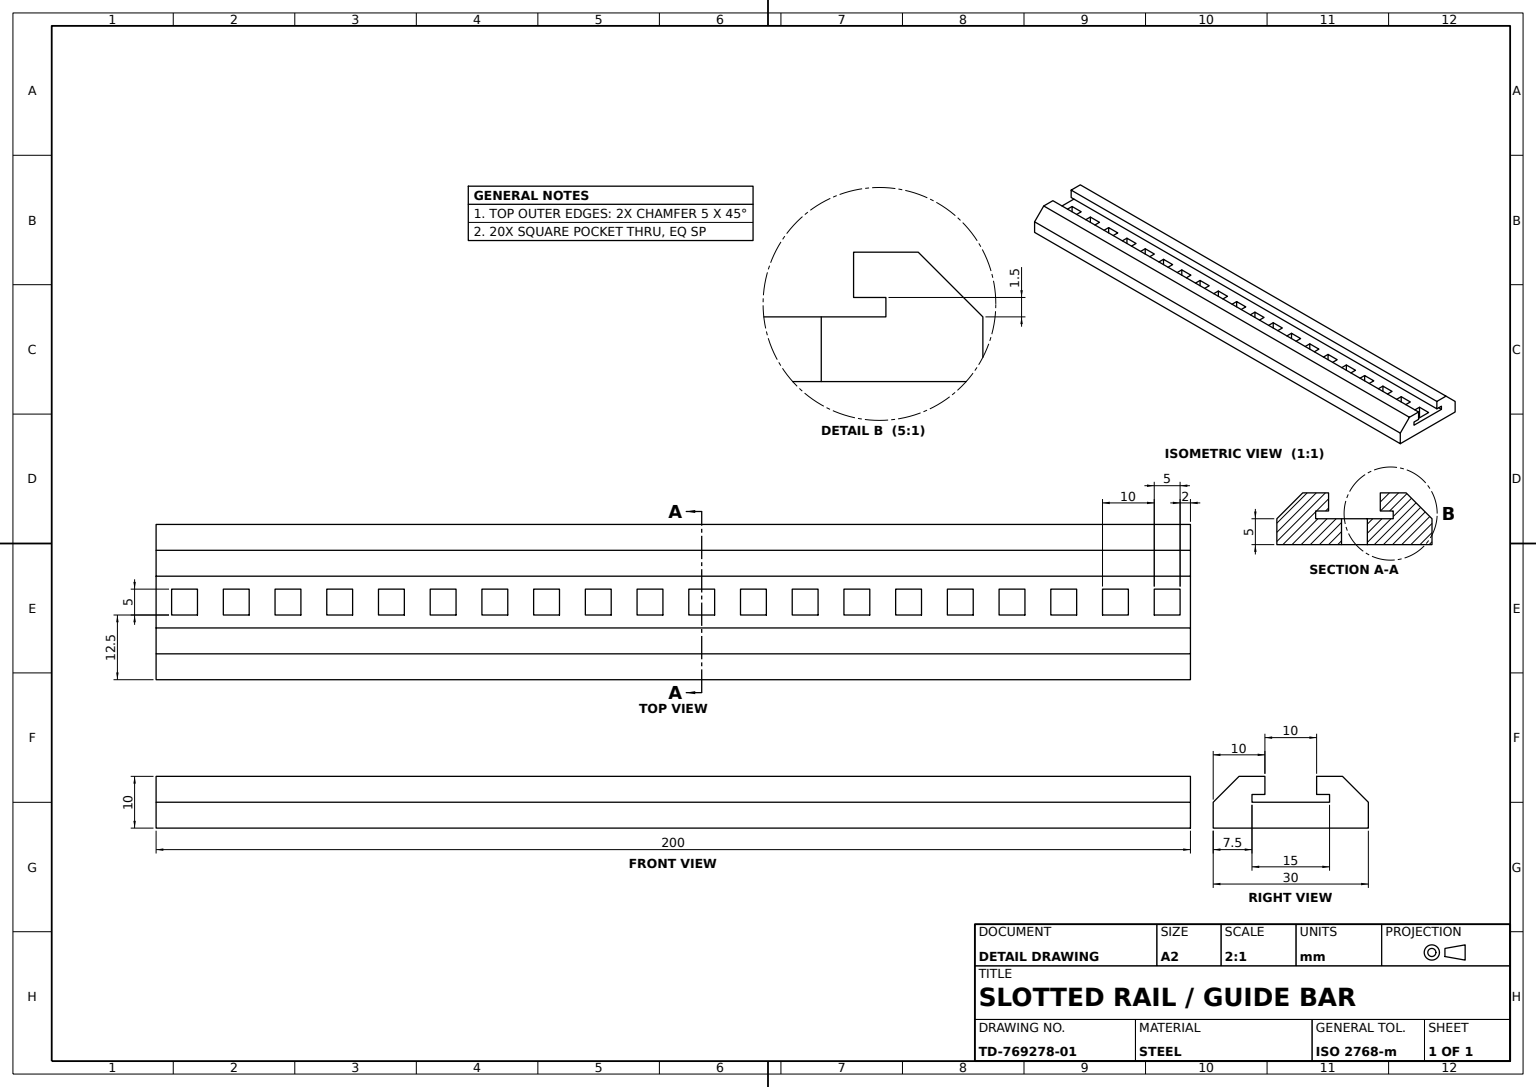
from build123d import *

# Parameters (mm, degrees)
TRACK_PROFILE_SKETCH_W            = 30
TRACK_PROFILE_SKETCH_H            = 10
TRACK_BODY_200MM_DEPTH            = 100
EDGE_CHAMFER_5MM_SIZE             = 5
GUIDE_GROOVE_SKETCH_W             = 10
GUIDE_GROOVE_SKETCH_H             = 200
GUIDE_GROOVE_10X5_DEPTH           = 5
END_START                         = -200
END_NOTCH_SKETCH_W                = 15
END_NOTCH_SKETCH_H                = 1.5
END_NOTCH_CUT_DEPTH               = 200
RACK_POCKET_CUT_REACH             = 103.242
RACK_POCKET_SKETCH_W              = 5
RACK_POCKET_SKETCH_H              = 5
RACK_POCKET_PATTERN_20X10MM_COUNT = 20
RACK_POCKET_PATTERN_20X10MM_PITCH = 10


with BuildPart() as part:
    # Track Profile Sketch → Track Body 200mm (new, symmetric)
    with BuildSketch(Plane.XY):
        Rectangle(TRACK_PROFILE_SKETCH_W, TRACK_PROFILE_SKETCH_H)
    extrude(amount=TRACK_BODY_200MM_DEPTH, both=True)

    # Edge Chamfer 5mm
    edge_chamfer_5mm_edges = [part.edges().sort_by_distance(p)[0] for p in [
        (-15, 5, 0),
        (15, 5, 0),
    ]]
    chamfer(edge_chamfer_5mm_edges, length=EDGE_CHAMFER_5MM_SIZE)

    # Guide Groove Sketch → Guide Groove 10x5 (cut)
    with BuildSketch(Plane(origin=(0, 5, 0), x_dir=(1, 0, 0), z_dir=(0, 1, 0))):
        Rectangle(GUIDE_GROOVE_SKETCH_W, GUIDE_GROOVE_SKETCH_H)
    extrude(amount=-GUIDE_GROOVE_10X5_DEPTH, mode=Mode.SUBTRACT)

    # End Notch Sketch → End Notch Cut (cut)
    with BuildSketch(Plane.XY.offset(100).offset(END_START)):
        with Locations((0, 0.75)):
            Rectangle(END_NOTCH_SKETCH_W, END_NOTCH_SKETCH_H)
    extrude(amount=END_NOTCH_CUT_DEPTH, mode=Mode.SUBTRACT)

    # Rack Pocket Sketch → Rack Pocket Cut (cut, up to next)
    with BuildSketch(Plane(origin=(0, 0, 0), x_dir=(1, 0, 0), z_dir=(0, 1, 0)), mode=Mode.PRIVATE) as rack_pocket_cut_sk1:
        with Locations((0, 95.5)):
            Rectangle(RACK_POCKET_SKETCH_W, RACK_POCKET_SKETCH_H)
    rack_pocket_cut_tool1 = extrude(rack_pocket_cut_sk1.sketch, amount=-RACK_POCKET_CUT_REACH, mode=Mode.PRIVATE) & part.part
    rack_pocket_cut = rack_pocket_cut_tool1.solids().sort_by_distance((0, 0, -95.5))[0]
    add(rack_pocket_cut, mode=Mode.SUBTRACT)

    # Rack Pocket Pattern 20x10mm: Rack Pocket Cut ×20
    with Locations(*[(0, 0, i * RACK_POCKET_PATTERN_20X10MM_PITCH) for i in range(1, RACK_POCKET_PATTERN_20X10MM_COUNT)]):
        add(rack_pocket_cut, mode=Mode.SUBTRACT)


solid = part.part
